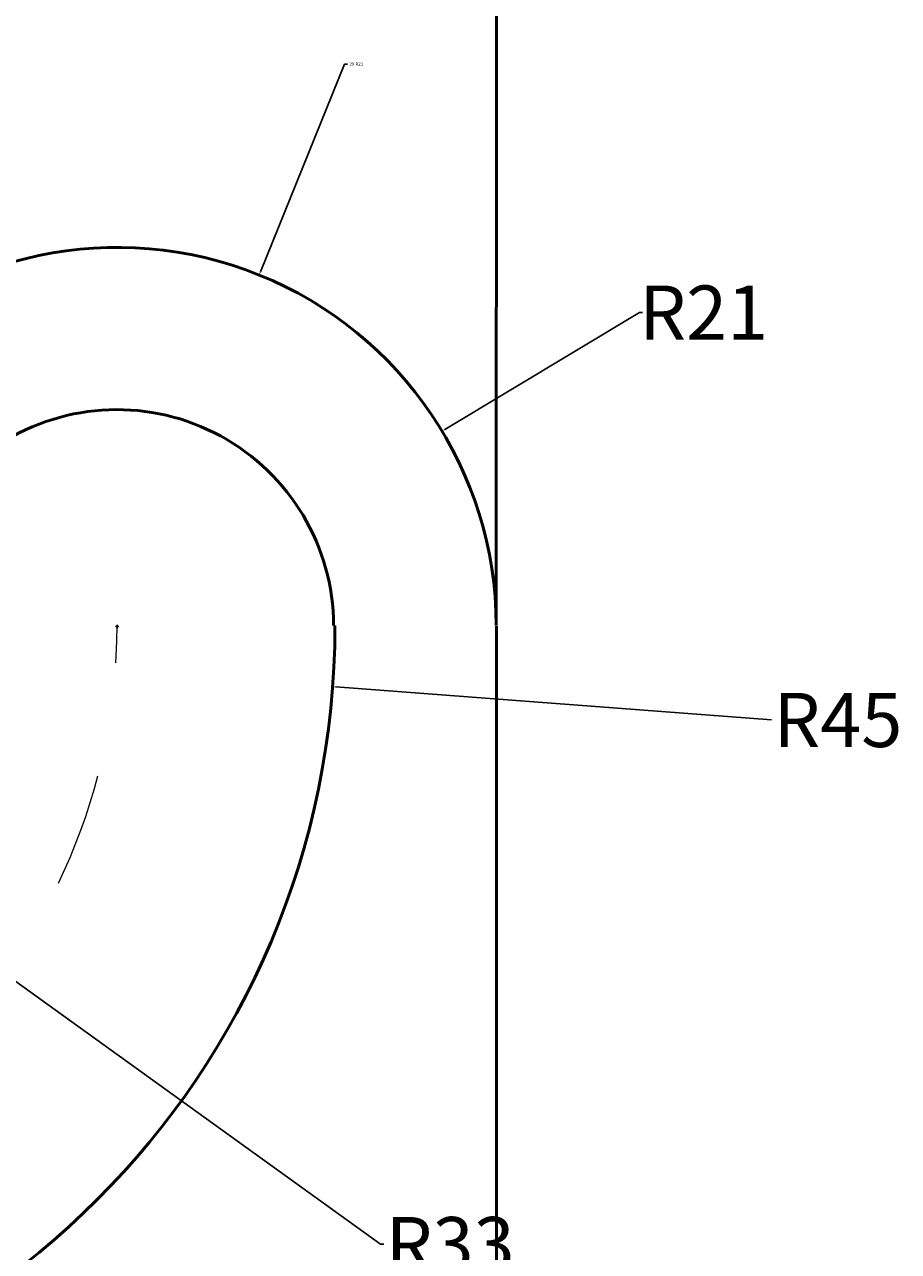
# Model space of a CAD drawing. Units: millimetres. Extents: x -50 to 109, y -46 to 152.
# Tile 14 of 18: x 61 to 109, y 32 to 100. Entities that reach past the tile are written whole.
import ezdxf

# ---------------------------------------------------------------- set-up
doc = ezdxf.new("R2010")
doc.units = ezdxf.units.MM
doc.header["$MEASUREMENT"] = 0
doc.linetypes.add('CENTER', pattern=[50.8, 31.75, -6.35, 6.35, -6.35])
for name, color, linetype, lineweight in [('M-CNTR', 1, 'CENTER', 18), ('M-DIMS', 2, 'Continuous', 25), ('M-OUTL', 7, 'Continuous', 50)]:
    doc.layers.add(name, color=color, linetype=linetype, lineweight=lineweight)
doc.styles.get("Standard").update_dxf_attribs({"font": 'arial.ttf'})
doc.dimstyles.get("Standard").update_dxf_attribs({"dimtxt": 0.18, "dimasz": 0.18, "dimexe": 0.18, "dimexo": 0.0625, "dimgap": 0.09, "dimtad": 0, "dimtih": 1, "dimtoh": 1, "dimdec": 4, "dimzin": 0, "dimdsep": 46, "dimtxsty": 'Standard', "dimcen": 0.09, "dimadec": 0, "dimazin": 0, "dimtfac": 1, "dimtdec": 4, "dimtofl": 0, "dimtmove": 0, "dimatfit": 3, "dimfxl": 1, "dimtolj": 1, "dimtzin": 0, "dimarcsym": 0})

# ---------------------------------------------------------------- blocks, each defined once
blk = doc.blocks.new('*D18')
at = {"layer": 'Defpoints', "color": 0, "transparency": 16777216}
for p in [(33.131, 66.25), (59.909, 46.965)]:
    blk.add_point(p, dxfattribs=at)
at = {"layer": 'M-DIMS', "color": 0, "lineweight": -2, "transparency": 16777216}
for p, q in [((33.041, 66.25), (33.221, 66.25)), ((33.131, 66.16), (33.131, 66.34)), ((80.717, 31.98), (60.055, 46.86)), ((80.897, 31.98), (80.717, 31.98))]:
    blk.add_line(p, q, dxfattribs=at)
at = {"layer": 'M-DIMS', "color": 0, "transparency": 16777216}
blk.add_solid([(60.073, 46.884), (60.038, 46.835), (59.909, 46.965)], dxfattribs=at)
at = {"layer": 'M-DIMS', "color": 0, "transparency": 16777216, "insert": (84.571, 31.98), "char_height": 0.18, "attachment_point": 5}
blk.add_mtext('\\A1;{\\H16.66667x;R33}', dxfattribs=at)
blk = doc.blocks.new('*D27')
at = {"layer": 'Defpoints', "color": 0, "transparency": 16777216}
for p in [(84.127, 77.003), (66.13, 66.182)]:
    blk.add_point(p, dxfattribs=at)
at = {"layer": 'M-DIMS', "color": 0, "lineweight": -2, "transparency": 16777216}
for p, q in [((95.051, 83.571), (84.282, 77.096)), ((95.231, 83.571), (95.051, 83.571)), ((66.04, 66.182), (66.22, 66.182)), ((66.13, 66.092), (66.13, 66.272))]:
    blk.add_line(p, q, dxfattribs=at)
at = {"layer": 'M-DIMS', "color": 0, "transparency": 16777216}
blk.add_solid([(84.266, 77.121), (84.297, 77.07), (84.127, 77.003)], dxfattribs=at)
at = {"layer": 'M-DIMS', "color": 0, "transparency": 16777216, "insert": (98.616, 83.571), "char_height": 0.18, "attachment_point": 5}
blk.add_mtext('\\A1;{\\H16.66667x;R21}', dxfattribs=at)
blk = doc.blocks.new('*D28')
at = {"layer": 'Defpoints', "color": 0, "transparency": 16777216}
for p in [(33.197, 66.25), (78.068, 62.85)]:
    blk.add_point(p, dxfattribs=at)
at = {"layer": 'M-DIMS', "color": 0, "lineweight": -2, "transparency": 16777216}
for p, q in [((33.107, 66.25), (33.287, 66.25)), ((33.197, 66.16), (33.197, 66.34)), ((102.361, 61.009), (78.248, 62.836))]:
    blk.add_line(p, q, dxfattribs=at)
at = {"layer": 'M-DIMS', "color": 0, "transparency": 16777216}
blk.add_solid([(78.25, 62.866), (78.246, 62.806), (78.068, 62.85)], dxfattribs=at)
at = {"layer": 'M-DIMS', "color": 0, "transparency": 16777216, "insert": (106.046, 61.009), "char_height": 0.18, "attachment_point": 5}
blk.add_mtext('\\A1;{\\H16.66667x;R45}', dxfattribs=at)
blk = doc.blocks.new('*D34')
at = {"layer": 'Defpoints', "color": 0, "transparency": 16777216}
for p in [(73.997, 85.653), (66.13, 66.182)]:
    blk.add_point(p, dxfattribs=at)
at = {"layer": 'M-DIMS', "color": 0, "lineweight": -2, "transparency": 16777216}
for p, q in [((78.717, 97.335), (74.064, 85.82)), ((78.897, 97.335), (78.717, 97.335)), ((66.04, 66.182), (66.22, 66.182)), ((66.13, 66.092), (66.13, 66.272))]:
    blk.add_line(p, q, dxfattribs=at)
at = {"layer": 'M-DIMS', "color": 0, "transparency": 16777216}
blk.add_solid([(74.037, 85.831), (74.092, 85.809), (73.997, 85.653)], dxfattribs=at)
at = {"layer": 'M-DIMS', "color": 0, "transparency": 16777216, "insert": (79.38, 97.335), "char_height": 0.18, "attachment_point": 5}
blk.add_mtext('\\A1;2X R21', dxfattribs=at)

msp = doc.modelspace()

# ---------------------------------------------------------------- linework, layer by layer
at = {"layer": 'M-CNTR'}
msp.add_arc((33.1307, 66.24997), 33, 180.0142817, 359.9857183, dxfattribs=at)
at = {"layer": 'M-OUTL'}
for p, q in [((87.1447, 114.19973), (87.12678, 66.54447)), ((78.12317, 66.24174), (78.197, 66.24174)), ((87.14026, 66.21184), (87.14026, 3.24112))]:
    msp.add_line(p, q, dxfattribs=at)
for centre, radius, start, end in [((66.1299, 66.18218), 21, 0.1625151, 135.8359859), ((66.12325, 66.19749), 12, 0.2112757, 183.9379291), ((33.197, 66.24997), 45, 180.0104732, 359.9895268)]:
    msp.add_arc(centre, radius, start, end, dxfattribs=at)

# ---------------------------------------------------------------- dimensions: what is measured, and where the dimension line sits
at = {"layer": 'M-DIMS'}
for center, mpoint, text, override, picture, middle in [((66.1299, 66.18218), (73.99696, 85.65291), '2X <>', {"dimdec": 0, "dimlfac": 1, "dimrnd": 0, "dimzin": 0, "dimdsep": 46, "dimlunit": 2}, '*D34', (79.3798, 97.33535)), ((66.1299, 66.18218), (84.12744, 77.00292), '{\\H16.66667x;R21}', {"dimclrd": 0, "dimclre": 0, "dimclrt": 0}, '*D27', (98.61616, 83.57083)), ((33.1307, 66.24997), (59.90911, 46.96483), '{\\H16.66667x;R33}', {"dimclrd": 0, "dimclre": 0, "dimclrt": 0}, '*D18', (84.57118, 31.97955)), ((33.197, 66.24997), (78.06836, 62.8499), '{\\H16.66667x;R45}', {"dimclrd": 0, "dimclre": 0, "dimclrt": 0}, '*D28', (102.36058, 61.0092))]:
    dim = msp.add_radius_dim(center=center, mpoint=mpoint, text=text, dimstyle='Standard', override=override, dxfattribs=at)
    dim.commit()
    dim.dimension.update_dxf_attribs({"geometry": picture, "text_midpoint": middle, "dimtype": 164})

doc.saveas('drawing.dxf')
